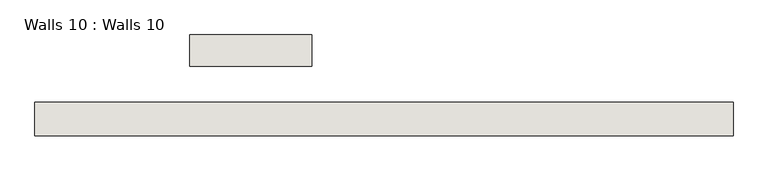
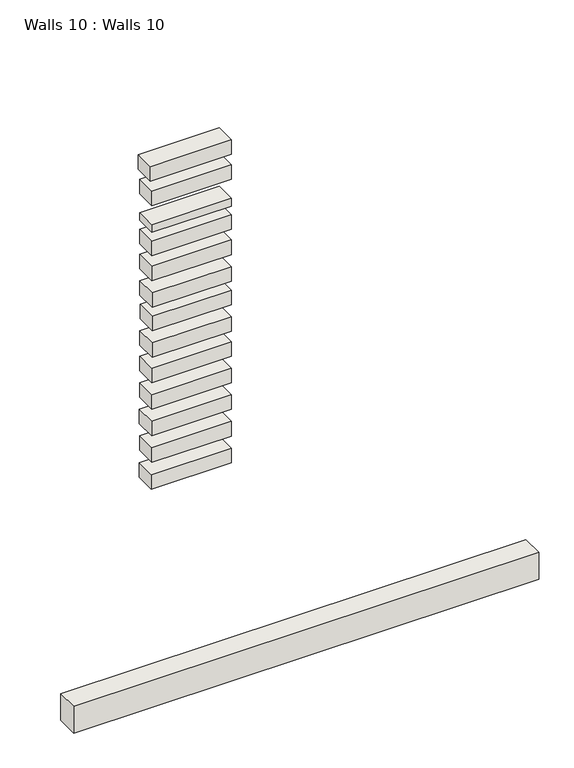
"""IFC4 building model written with IfcOpenShell, lengths in millimetres: wall geometry, Walls 10 : Walls 10."""

from ifc_helpers import new_model, si_unit, frame, origin, place, context, project, spatial, polyline, outline, extrude, source, transform, mapped, element, save


def walls_10_walls_10_12dc5ecd(model_context):
    return source(origin(), model_context, "Body", "SweptSolid", [
        extrude(outline(polyline([(-8250.7305193, -4624.7687977), (-15391.5925702, -4624.7687977), (-15391.5925702, -4285.7213241), (-8250.7305193, -4285.7213241), (-8250.7305193, -4624.7687977)])), frame((0.0, 0.0, 1238.4931347), z_axis=(0.0, 0.0, 1.0), x_axis=(1.0, 0.0, 0.0)), (0.0, 0.0, 1.0), 437.0057515),
        extrude(outline(polyline([(-12560.3288845, -3916.9259649), (-13805.7728698, -3916.9259649), (-13805.7728698, -3595.8286913), (-12560.3288845, -3595.8286913), (-12560.3288845, -3916.9259649)])), frame((0.0, 0.0, 9212.8470483), z_axis=(0.0, 0.0, 1.0), x_axis=(1.0, 0.0, 0.0)), (0.0, 0.0, 1.0), 235.9529517),
        extrude(outline(polyline([(-12560.3288845, -3916.9259649), (-13781.1017742, -3916.9259649), (-13781.1017742, -3595.8286913), (-12560.3288845, -3595.8286913), (-12560.3288845, -3916.9259649)])), frame((0.0, 0.0, 8806.4470483), z_axis=(0.0, 0.0, 1.0), x_axis=(1.0, 0.0, 0.0)), (0.0, 0.0, 1.0), 235.9529517),
        extrude(outline(polyline([(-12560.3288845, -3916.9259649), (-13783.9399214, -3916.9259649), (-13783.9399214, -3595.8286913), (-12560.3288845, -3595.8286913), (-12560.3288845, -3916.9259649)])), frame((0.0, 0.0, 8374.6470483), z_axis=(0.0, 0.0, 1.0), x_axis=(1.0, 0.0, 0.0)), (0.0, 0.0, 1.0), 125.4305895),
        extrude(outline(polyline([(-12560.3288845, -3916.9259649), (-13782.6613762, -3916.9259649), (-13782.6613762, -3595.8286913), (-12560.3288845, -3595.8286913), (-12560.3288845, -3916.9259649)])), frame((0.0, 0.0, 7993.6470483), z_axis=(0.0, 0.0, 1.0), x_axis=(1.0, 0.0, 0.0)), (0.0, 0.0, 1.0), 235.9529517),
        extrude(outline(polyline([(-12560.3288845, -3916.9259649), (-13783.5482518, -3916.9259649), (-13783.5482518, -3595.8286913), (-12560.3288845, -3595.8286913), (-12560.3288845, -3916.9259649)])), frame((0.0, 0.0, 7587.2470483), z_axis=(0.0, 0.0, 1.0), x_axis=(1.0, 0.0, 0.0)), (0.0, 0.0, 1.0), 235.9529517),
        extrude(outline(polyline([(-12560.3288845, -3916.9259649), (-13778.4968347, -3916.9259649), (-13778.4968347, -3595.8286913), (-12560.3288845, -3595.8286913), (-12560.3288845, -3916.9259649)])), frame((0.0, 0.0, 7155.4470483), z_axis=(0.0, 0.0, 1.0), x_axis=(1.0, 0.0, 0.0)), (0.0, 0.0, 1.0), 235.9529517),
        extrude(outline(polyline([(-12560.3288845, -3916.9259649), (-13775.6172167, -3916.9259649), (-13775.6172167, -3595.8286913), (-12560.3288845, -3595.8286913), (-12560.3288845, -3916.9259649)])), frame((0.0, 0.0, 6774.4470483), z_axis=(0.0, 0.0, 1.0), x_axis=(1.0, 0.0, 0.0)), (0.0, 0.0, 1.0), 235.9529517),
        extrude(outline(polyline([(-12560.3288845, -3916.9259649), (-13778.2116586, -3916.9259649), (-13778.2116586, -3595.8286913), (-12560.3288845, -3595.8286913), (-12560.3288845, -3916.9259649)])), frame((0.0, 0.0, 6342.6470483), z_axis=(0.0, 0.0, 1.0), x_axis=(1.0, 0.0, 0.0)), (0.0, 0.0, 1.0), 235.9529517),
        extrude(outline(polyline([(-12560.3288845, -3916.9259649), (-13784.9020016, -3916.9259649), (-13784.9020016, -3595.8286913), (-12560.3288845, -3595.8286913), (-12560.3288845, -3916.9259649)])), frame((0.0, 0.0, 5936.2470483), z_axis=(0.0, 0.0, 1.0), x_axis=(1.0, 0.0, 0.0)), (0.0, 0.0, 1.0), 235.9529517),
        extrude(outline(polyline([(-12560.3288845, -3916.9259649), (-13782.572219, -3916.9259649), (-13782.572219, -3595.8286913), (-12560.3288845, -3595.8286913), (-12560.3288845, -3916.9259649)])), frame((0.0, 0.0, 5504.4470483), z_axis=(0.0, 0.0, 1.0), x_axis=(1.0, 0.0, 0.0)), (0.0, 0.0, 1.0), 235.9529517),
        extrude(outline(polyline([(-12560.3288845, -3916.9259649), (-13786.5392482, -3916.9259649), (-13786.5392482, -3595.8286913), (-12560.3288845, -3595.8286913), (-12560.3288845, -3916.9259649)])), frame((0.0, 0.0, 5072.6470483), z_axis=(0.0, 0.0, 1.0), x_axis=(1.0, 0.0, 0.0)), (0.0, 0.0, 1.0), 235.9529517),
        extrude(outline(polyline([(-12560.3288845, -3916.9259649), (-13780.7547871, -3916.9259649), (-13780.7547871, -3595.8286913), (-12560.3288845, -3595.8286913), (-12560.3288845, -3916.9259649)])), frame((0.0, 0.0, 4640.8470483), z_axis=(0.0, 0.0, 1.0), x_axis=(1.0, 0.0, 0.0)), (0.0, 0.0, 1.0), 235.9529517),
        extrude(outline(polyline([(-12560.3288845, -3916.9259649), (-13790.8727167, -3916.9259649), (-13790.8727167, -3595.8286913), (-12560.3288845, -3595.8286913), (-12560.3288845, -3916.9259649)])), frame((0.0, 0.0, 4209.0470483), z_axis=(0.0, 0.0, 1.0), x_axis=(1.0, 0.0, 0.0)), (0.0, 0.0, 1.0), 235.9529517),
    ])


if __name__ == "__main__":
    model = new_model("IFC4")
    model_context = context("Model", 3, world=origin())
    ifc_project = project(units=[si_unit("LENGTHUNIT", "METRE", prefix="MILLI")], contexts=[model_context])
    site = spatial("IfcSite", under=ifc_project)
    building = spatial("IfcBuilding", under=site)
    placement = place(None, origin())
    walls_10_walls_10_shape = walls_10_walls_10_12dc5ecd(model_context)
    element("IfcWall", 1, ObjectType="Walls 10 : Walls 10", at=placement, inside=building, context=model_context, shape_type="MappedRepresentation", body=[
        mapped(walls_10_walls_10_shape, transform((0.0, 0.0, 0.0), x_axis=(1.0, 0.0, 0.0), y_axis=(0.0, 1.0, 0.0), z_axis=(0.0, 0.0, 1.0))),
    ])
    save(model, "model.ifc")

# Revit data of these elements
# Element 1 (IfcWall, "Walls 10 : Walls 10")
#   Materials on its faces: "Default Wall"
# Materials
#   "Default Wall": colour RGB 128 128 128, transparency 0
